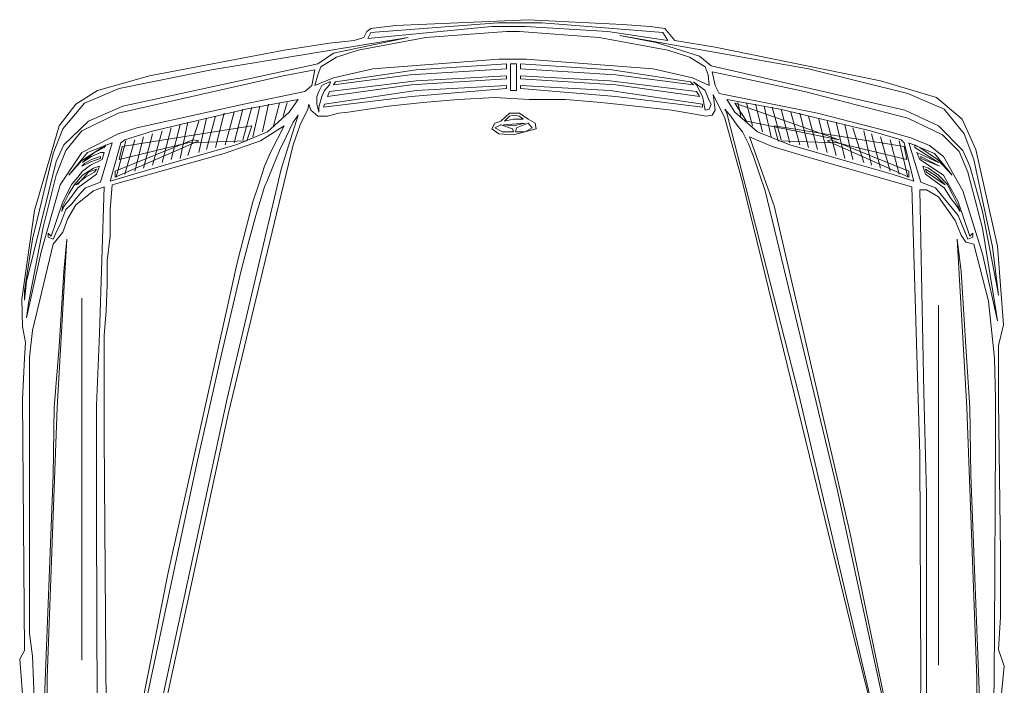
# Model space of a CAD drawing. Units: inches. Extents: x -9 to 646, y -802 to 47.
# Tile 9 of 17: x 432 to 486, y -561 to -525. Entities that reach past the tile are written whole.
import ezdxf

# ---------------------------------------------------------------- set-up
doc = ezdxf.new("R2010")
doc.units = ezdxf.units.IN
doc.header["$MEASUREMENT"] = 0
doc.layers.add('A-SITE-VEHI', color=8, linetype='Continuous', lineweight=9)

msp = doc.modelspace()

# ---------------------------------------------------------------- linework, layer by layer
at = {"layer": 'A-SITE-VEHI'}
for p, q in [((457.811, -525.081), (450.981, -525.732)), ((451.143, -525.408), (458.135, -524.866)), ((452.5, -525.028), (451.143, -525.19)), ((459.816, -524.701), (452.5, -525.028)), ((459.654, -525.081), (457.811, -525.081)), ((458.135, -524.866), (460.575, -524.866)), ((464.206, -525.352), (459.654, -525.081)), ((465.019, -524.974), (459.816, -524.701)), ((460.575, -524.866), (467.241, -525.408)), ((466.537, -525.081), (465.019, -524.974)), ((467.35, -525.19), (466.537, -525.081)), ((442.363, -527.466), (453.204, -525.678)), ((453.204, -525.678), (449.085, -526.544)), ((450.763, -525.678), (450.222, -525.841)), ((450.439, -526.382), (454.178, -525.678)), ((450.928, -525.352), (450.763, -525.678)), ((451.143, -525.19), (450.928, -525.352)), ((450.981, -525.732), (451.143, -525.408)), ((454.178, -525.678), (458.624, -525.352)), ((458.624, -525.352), (459.328, -525.352)), ((459.328, -525.352), (463.717, -525.678)), ((463.717, -525.678), (467.512, -526.382)), ((467.512, -525.841), (464.206, -525.352)), ((475.264, -527.413), (464.856, -525.57)), ((464.856, -525.57), (466.862, -525.949)), ((467.241, -525.408), (467.512, -525.841)), ((467.892, -525.841), (467.35, -525.19)), ((448.867, -526.003), (446.374, -526.382)), ((450.222, -525.841), (448.867, -526.003)), ((466.862, -525.949), (469.246, -526.709)), ((470.114, -526.22), (467.892, -525.841)), ((479.221, -528.063), (470.114, -526.22)), ((446.374, -526.382), (438.948, -527.792)), ((449.085, -526.544), (448.216, -527.142)), ((448.379, -527.304), (449.247, -526.762)), ((449.247, -526.762), (450.439, -526.382)), ((467.512, -526.382), (468.705, -526.762)), ((468.705, -526.762), (469.573, -527.304)), ((469.246, -526.709), (469.897, -527.25)), ((448.216, -527.142), (437.485, -529.473)), ((448.216, -527.737), (448.379, -527.304)), ((458.191, -526.871), (451.252, -527.413)), ((453.637, -527.466), (458.624, -527.142)), ((459.707, -526.871), (458.191, -526.871)), ((458.624, -527.142), (458.624, -527.413)), ((459.165, -527.142), (458.841, -527.142)), ((458.841, -527.142), (458.841, -528.605)), ((459.165, -528.605), (459.165, -527.142)), ((464.423, -527.466), (459.383, -527.142)), ((459.383, -527.142), (459.383, -527.413)), ((466.699, -527.413), (459.707, -526.871)), ((469.573, -527.304), (469.735, -527.737)), ((469.897, -527.25), (480.575, -529.689)), ((438.948, -527.792), (436.075, -528.605)), ((437.214, -529.851), (446.32, -527.792)), ((437.267, -528.496), (442.363, -527.466)), ((446.32, -527.792), (448.054, -527.466)), ((448.054, -527.466), (447.892, -528.334)), ((448.054, -528.334), (448.216, -527.737)), ((451.252, -527.413), (449.085, -527.901)), ((453.312, -527.737), (449.085, -528.281)), ((449.193, -528.116), (453.637, -527.466)), ((458.624, -527.413), (453.312, -527.737)), ((453.637, -528.063), (458.624, -527.792)), ((458.624, -527.792), (458.624, -527.954)), ((459.383, -527.413), (464.639, -527.737)), ((464.315, -528.063), (459.383, -527.792)), ((459.383, -527.792), (459.383, -527.954)), ((468.76, -528.116), (464.423, -527.466)), ((464.639, -527.737), (468.922, -528.281)), ((468.867, -527.901), (466.699, -527.413)), ((469.735, -527.737), (469.788, -528.334)), ((471.524, -527.901), (469.952, -527.575)), ((469.952, -527.575), (470.114, -528.334)), ((480.737, -528.767), (475.264, -527.413)), ((447.892, -528.334), (447.513, -528.658)), ((449.085, -527.901), (448.054, -528.334)), ((448.434, -528.334), (448.272, -528.658)), ((448.867, -528.116), (448.434, -528.334)), ((448.596, -528.605), (448.867, -528.281)), ((453.366, -528.281), (448.758, -528.929)), ((448.867, -528.658), (453.637, -528.063)), ((448.867, -528.281), (448.923, -528.116)), ((448.923, -528.116), (448.867, -528.116)), ((449.085, -528.281), (449.193, -528.116)), ((458.624, -527.954), (453.366, -528.281)), ((453.637, -528.605), (458.624, -528.334)), ((458.624, -528.334), (458.624, -528.496)), ((459.383, -527.954), (464.639, -528.281)), ((464.315, -528.605), (459.383, -528.334)), ((459.383, -528.334), (459.383, -528.496)), ((469.084, -528.658), (464.315, -528.063)), ((464.639, -528.281), (469.246, -528.929)), ((468.922, -528.281), (468.76, -528.116)), ((469.788, -528.334), (468.867, -527.901)), ((469.573, -528.605), (468.922, -528.116)), ((468.922, -528.116), (469.084, -528.281)), ((469.084, -528.281), (469.411, -528.929)), ((470.114, -528.334), (470.332, -528.767)), ((475.046, -528.658), (471.524, -527.901)), ((482.309, -528.985), (479.221, -528.063)), ((436.075, -528.605), (434.883, -529.364)), ((435.371, -529.309), (437.267, -528.496)), ((447.513, -528.658), (444.151, -529.364)), ((448.272, -528.658), (448.163, -528.929)), ((448.163, -528.929), (448.163, -529.364)), ((448.272, -529.526), (448.434, -528.929)), ((448.434, -528.929), (448.596, -528.605)), ((453.366, -528.929), (448.543, -529.526)), ((448.596, -529.364), (453.637, -528.605)), ((448.758, -528.929), (448.867, -528.658)), ((458.624, -528.496), (453.366, -528.929)), ((458.841, -528.605), (459.165, -528.605)), ((459.383, -528.496), (464.639, -528.929)), ((469.411, -529.364), (464.315, -528.605)), ((464.639, -528.929), (469.411, -529.526)), ((469.246, -528.929), (469.084, -528.658)), ((469.411, -528.929), (469.573, -529.689)), ((469.788, -529.147), (469.573, -528.605)), ((470.656, -530.122), (470.006, -528.823)), ((470.006, -528.823), (470.114, -529.689)), ((470.332, -528.767), (475.752, -529.851)), ((480.737, -530.122), (475.046, -528.658)), ((482.742, -529.635), (480.737, -528.767)), ((434.883, -529.364), (433.961, -530.557)), ((434.179, -530.719), (435.371, -529.309)), ((437.485, -529.473), (435.589, -530.286)), ((444.151, -529.364), (438.244, -530.666)), ((444.26, -529.635), (447.133, -529.093)), ((444.639, -531.152), (445.019, -529.473)), ((445.181, -530.881), (445.507, -529.364)), ((445.778, -530.557), (446.103, -529.309)), ((446.32, -530.015), (446.538, -529.256)), ((447.133, -529.093), (446.644, -529.797)), ((447.73, -529.364), (447.675, -529.635)), ((447.837, -529.689), (447.73, -529.364)), ((448.163, -529.364), (448.272, -529.797)), ((448.543, -529.526), (448.596, -529.364)), ((452.12, -529.473), (449.897, -529.797)), ((454.016, -529.256), (452.12, -529.473)), ((455.968, -529.093), (454.016, -529.256)), ((457.973, -528.985), (455.968, -529.093)), ((459.869, -529.093), (457.973, -528.985)), ((461.877, -529.093), (459.869, -529.093)), ((463.826, -529.256), (461.877, -529.093)), ((465.725, -529.473), (463.826, -529.256)), ((467.73, -529.689), (465.725, -529.473)), ((469.411, -529.526), (469.411, -529.364)), ((469.897, -529.364), (469.788, -529.147)), ((469.788, -529.635), (469.897, -529.364)), ((473.692, -529.635), (470.765, -529.093)), ((470.765, -529.093), (471.198, -529.797)), ((476.945, -531.314), (471.198, -529.309)), ((471.198, -529.309), (471.849, -530.286)), ((471.524, -530.015), (471.36, -529.256)), ((472.173, -530.557), (471.849, -529.309)), ((472.717, -530.881), (472.337, -529.364)), ((473.203, -531.152), (472.823, -529.473)), ((483.719, -530.177), (482.309, -528.985)), ((435.209, -530.828), (437.214, -529.851)), ((439.166, -530.828), (444.26, -529.635)), ((442.092, -531.858), (442.581, -530.015)), ((442.581, -531.749), (443.067, -529.851)), ((443.123, -531.587), (443.609, -529.797)), ((443.609, -531.478), (444.098, -529.635)), ((444.098, -531.314), (444.586, -529.526)), ((446.644, -529.797), (445.452, -530.881)), ((446.211, -532.941), (447.133, -529.959)), ((447.133, -529.959), (446.862, -530.339)), ((447.675, -529.635), (447.242, -530.501)), ((448.216, -530.015), (447.837, -529.689)), ((448.758, -530.015), (448.216, -530.015)), ((448.272, -529.797), (448.272, -529.526)), ((449.356, -529.851), (448.758, -530.015)), ((449.897, -529.797), (449.356, -529.851)), ((458.786, -529.851), (458.297, -530.286)), ((458.786, -530.015), (458.515, -530.286)), ((459.328, -529.851), (458.786, -529.851)), ((459.003, -529.959), (458.786, -530.015)), ((459.328, -530.015), (459.003, -529.959)), ((459.816, -530.177), (459.328, -529.851)), ((459.545, -530.177), (459.328, -530.015)), ((469.626, -530.015), (467.73, -529.689)), ((469.573, -529.689), (469.788, -529.635)), ((469.952, -529.959), (469.626, -530.015)), ((470.114, -529.689), (469.952, -529.959)), ((470.981, -530.015), (470.656, -529.635)), ((470.656, -529.635), (470.765, -529.851)), ((470.765, -529.851), (474.722, -545.354)), ((471.307, -530.501), (470.981, -530.015)), ((471.198, -529.797), (472.444, -530.881)), ((473.745, -531.314), (473.259, -529.526)), ((478.679, -530.828), (473.692, -529.635)), ((474.233, -531.478), (473.745, -529.635)), ((474.775, -531.587), (474.287, -529.797)), ((475.264, -531.749), (474.775, -529.851)), ((475.752, -531.858), (475.264, -530.015)), ((475.752, -529.851), (479.545, -530.828)), ((480.575, -529.689), (482.418, -530.557)), ((483.828, -530.99), (482.742, -529.635)), ((433.961, -530.557), (432.607, -535.217)), ((435.589, -530.286), (434.232, -531.587)), ((437.432, -531.694), (444.586, -530.557)), ((440.141, -532.4), (440.629, -530.501)), ((440.629, -532.344), (441.062, -530.339)), ((441.062, -532.182), (441.659, -530.286)), ((441.659, -532.02), (442.092, -530.122)), ((444.586, -530.557), (444.315, -531.369)), ((446.374, -530.557), (445.072, -531.369)), ((445.616, -532.02), (446.374, -530.557)), ((446.862, -530.339), (446.482, -531.152)), ((447.242, -530.501), (446.862, -531.587)), ((457.973, -530.395), (457.811, -530.719)), ((458.297, -530.286), (457.973, -530.395)), ((458.297, -530.501), (457.973, -530.666)), ((458.948, -530.719), (458.297, -530.501)), ((459.654, -530.395), (458.462, -530.501)), ((458.462, -530.501), (459.003, -530.557)), ((458.515, -530.286), (459.003, -530.177)), ((459.003, -530.177), (459.545, -530.177)), ((459.003, -530.557), (459.654, -530.395)), ((459.816, -530.395), (459.165, -530.666)), ((460.196, -530.395), (459.816, -530.177)), ((460.034, -530.666), (459.816, -530.395)), ((460.249, -530.719), (460.196, -530.395)), ((471.631, -533.645), (470.656, -530.122)), ((471.631, -530.881), (471.307, -530.501)), ((471.849, -530.286), (476.945, -531.314)), ((480.522, -531.694), (473.365, -530.557)), ((473.365, -530.557), (473.583, -531.369)), ((476.294, -532.02), (475.806, -530.122)), ((476.78, -532.182), (476.294, -530.286)), ((477.269, -532.344), (476.78, -530.339)), ((477.702, -532.4), (477.269, -530.501)), ((482.636, -531.043), (480.737, -530.122)), ((482.418, -530.557), (483.772, -531.911)), ((484.479, -531.858), (483.719, -530.177)), ((433.637, -532.073), (434.179, -530.719)), ((434.341, -531.911), (435.209, -530.828)), ((437.214, -530.99), (435.209, -532.02)), ((438.244, -530.666), (437.214, -530.99)), ((437.594, -531.314), (439.166, -530.828)), ((438.624, -532.886), (439.11, -530.99)), ((439.11, -532.724), (439.652, -530.828)), ((439.652, -532.562), (440.141, -530.666)), ((445.452, -530.881), (443.718, -531.587)), ((457.811, -530.719), (458.191, -530.99)), ((457.973, -530.666), (458.406, -530.881)), ((458.191, -530.99), (459.003, -531.043)), ((458.406, -530.881), (459.003, -530.881)), ((459.003, -530.881), (458.948, -530.719)), ((459.003, -531.043), (460.249, -530.719)), ((459.165, -530.666), (459.112, -530.881)), ((459.112, -530.881), (459.654, -530.881)), ((459.654, -530.881), (460.034, -530.666)), ((471.957, -531.532), (471.631, -530.881)), ((472.444, -530.881), (474.233, -531.587)), ((478.299, -532.562), (477.702, -530.666)), ((478.732, -532.724), (478.299, -530.828)), ((480.357, -531.314), (478.679, -530.828)), ((479.221, -532.886), (478.732, -530.99)), ((479.545, -530.828), (480.899, -531.207)), ((483.557, -531.965), (482.636, -531.043)), ((484.37, -532.4), (483.828, -530.99)), ((434.232, -531.587), (433.799, -532.506)), ((435.533, -532.02), (436.89, -531.478)), ((436.89, -531.478), (436.239, -533.645)), ((436.564, -531.587), (436.346, -531.749)), ((436.455, -531.749), (436.564, -531.587)), ((436.781, -533.592), (437.376, -531.478)), ((437.052, -533.05), (441.333, -531.314)), ((441.659, -531.369), (437.052, -533.374)), ((437.105, -533.374), (437.647, -531.369)), ((441.062, -531.478), (437.267, -532.4)), ((437.376, -531.478), (437.594, -531.314)), ((437.594, -533.212), (438.136, -531.314)), ((438.136, -533.05), (438.624, -531.152)), ((443.718, -531.587), (440.467, -532.506)), ((444.315, -531.369), (441.062, -531.478)), ((441.333, -531.314), (441.659, -531.369)), ((445.072, -531.369), (443.067, -532.073)), ((446.862, -531.587), (443.285, -546.437)), ((446.482, -531.152), (446.103, -531.911)), ((472.228, -532.235), (471.957, -531.532)), ((473.259, -531.694), (472.011, -531.152)), ((472.011, -531.152), (473.365, -534.947)), ((473.583, -531.369), (476.836, -531.478)), ((474.233, -531.587), (477.431, -532.506)), ((476.509, -531.314), (476.294, -531.369)), ((476.294, -531.369), (480.793, -533.374)), ((480.793, -533.05), (476.509, -531.314)), ((476.836, -531.478), (480.684, -532.4)), ((479.762, -533.05), (479.221, -531.152)), ((480.251, -533.212), (479.762, -531.314)), ((480.737, -533.374), (480.251, -531.369)), ((480.522, -531.478), (480.357, -531.314)), ((481.064, -533.592), (480.522, -531.478)), ((482.2, -532.073), (480.793, -531.478)), ((480.793, -531.478), (481.443, -533.645)), ((480.899, -531.207), (481.93, -531.64)), ((481.117, -531.749), (481.117, -531.587)), ((481.117, -531.587), (481.388, -531.749)), ((481.93, -531.64), (482.689, -532.235)), ((432.498, -536.79), (433.637, -532.073)), ((433.799, -533.266), (434.341, -531.911)), ((435.209, -532.02), (434.017, -533.808)), ((434.503, -533.266), (435.533, -532.02)), ((436.346, -531.749), (435.209, -532.453)), ((435.751, -532.235), (435.262, -532.562)), ((435.425, -532.4), (435.913, -532.02)), ((436.239, -532.02), (435.751, -532.235)), ((435.751, -532.4), (436.239, -532.235)), ((435.913, -532.02), (436.455, -531.749)), ((436.455, -532.02), (436.239, -532.02)), ((436.239, -532.235), (436.239, -532.344)), ((436.346, -532.4), (436.455, -532.02)), ((443.067, -532.073), (436.89, -533.808)), ((437.267, -532.4), (437.432, -531.694)), ((445.29, -532.779), (445.616, -532.02)), ((446.103, -531.911), (445.778, -532.724)), ((472.553, -533.212), (472.228, -532.235)), ((475.479, -532.344), (473.259, -531.694)), ((480.684, -532.4), (480.522, -531.694)), ((482.418, -532.562), (481.117, -531.749)), ((481.388, -532.4), (481.226, -532.02)), ((481.226, -532.02), (482.418, -532.562)), ((481.388, -531.749), (482.365, -532.4)), ((481.443, -532.235), (481.443, -532.344)), ((482.471, -532.779), (481.443, -532.235)), ((483.177, -533.266), (482.2, -532.073)), ((482.689, -532.235), (483.772, -534.134)), ((484.043, -533.104), (483.557, -531.965)), ((483.772, -531.911), (484.152, -532.779)), ((485.671, -537.169), (484.479, -531.858)), ((433.799, -532.506), (432.174, -539.121)), ((435.209, -532.453), (434.503, -533.266)), ((435.751, -532.506), (435.209, -532.779)), ((435.209, -532.779), (435.371, -532.615)), ((435.262, -532.562), (435.425, -532.4)), ((435.262, -533.05), (435.698, -532.724)), ((435.371, -532.615), (435.751, -532.4)), ((435.698, -532.724), (436.346, -532.4)), ((436.239, -532.344), (435.751, -532.506)), ((440.467, -532.506), (438.082, -533.212)), ((445.778, -532.724), (445.452, -533.537)), ((480.955, -533.916), (475.479, -532.344)), ((477.431, -532.506), (479.871, -533.212)), ((482.689, -533.266), (481.388, -532.4)), ((481.443, -532.344), (482.471, -532.779)), ((482.365, -532.4), (483.177, -533.266)), ((485.398, -537.223), (484.37, -532.4)), ((433.095, -536.139), (433.799, -533.266)), ((434.829, -533.754), (435.262, -533.266)), ((434.991, -533.374), (435.262, -533.05)), ((434.991, -533.754), (435.589, -533.104)), ((436.022, -533.212), (434.991, -533.972)), ((435.262, -533.266), (435.86, -532.886)), ((435.913, -533.104), (435.425, -533.374)), ((435.589, -533.104), (436.022, -532.941)), ((435.86, -532.886), (436.184, -532.779)), ((436.022, -532.941), (435.913, -533.104)), ((436.184, -532.779), (436.022, -533.212)), ((438.082, -533.212), (436.781, -533.592)), ((437.052, -533.374), (437.052, -533.05)), ((443.232, -545.569), (446.211, -532.941)), ((444.966, -533.754), (445.29, -532.779)), ((472.879, -534.134), (472.553, -533.212)), ((479.871, -533.212), (481.064, -533.592)), ((480.793, -533.374), (480.793, -533.05)), ((481.876, -532.886), (481.55, -532.779)), ((481.55, -532.779), (481.714, -533.212)), ((482.309, -533.321), (481.714, -532.941)), ((481.714, -532.941), (481.767, -533.104)), ((481.714, -533.212), (482.742, -533.972)), ((481.767, -533.104), (482.798, -533.808)), ((482.418, -533.266), (481.876, -532.886)), ((482.906, -533.754), (482.418, -533.266)), ((483.502, -534.729), (482.689, -533.266)), ((484.856, -536.192), (484.043, -533.104)), ((484.152, -532.779), (484.856, -535.271)), ((434.017, -533.808), (432.986, -537.493)), ((434.179, -534.729), (434.667, -533.754)), ((434.503, -534.296), (434.829, -533.754)), ((434.667, -533.754), (434.991, -533.374)), ((435.425, -533.374), (434.883, -533.808)), ((434.883, -533.808), (434.991, -533.754)), ((435.86, -533.808), (435.425, -533.972)), ((436.239, -533.645), (435.86, -533.808)), ((436.89, -533.808), (436.781, -535.164)), ((444.639, -534.729), (444.966, -533.754)), ((445.452, -533.537), (445.29, -533.916)), ((474.287, -544.541), (471.631, -533.645)), ((481.443, -533.645), (482.256, -533.972)), ((482.798, -533.808), (482.309, -533.321)), ((483.177, -534.296), (482.906, -533.754)), ((434.179, -534.947), (434.503, -534.296)), ((434.991, -533.972), (434.558, -534.567)), ((435.86, -534.134), (434.883, -534.893)), ((435.154, -534.243), (434.883, -534.567)), ((435.425, -533.972), (435.154, -534.243)), ((436.455, -533.916), (435.86, -534.134)), ((436.184, -541.992), (436.455, -533.916)), ((445.29, -533.916), (444.801, -535.488)), ((476.836, -550.556), (472.879, -534.134)), ((481.388, -548.66), (480.955, -533.916)), ((481.767, -534.078), (481.388, -534.078)), ((481.388, -534.078), (481.605, -545.245)), ((482.418, -534.458), (481.767, -534.078)), ((482.256, -533.972), (483.502, -535.488)), ((482.742, -533.972), (483.122, -534.567)), ((483.502, -534.947), (483.177, -534.296)), ((483.772, -534.134), (484.856, -537.602)), ((433.799, -535.815), (434.179, -534.729)), ((434.125, -535.271), (434.179, -534.947)), ((434.558, -534.567), (434.232, -535)), ((434.667, -534.838), (434.341, -535.164)), ((434.883, -534.893), (434.45, -535.65)), ((434.883, -534.567), (434.667, -534.838)), ((444.315, -536.03), (444.639, -534.729)), ((473.365, -534.947), (477.54, -552.941)), ((483.339, -535.759), (482.418, -534.458)), ((483.122, -534.567), (483.448, -535)), ((484.152, -536.627), (483.502, -534.729)), ((483.61, -535.271), (483.502, -534.947)), ((432.607, -535.217), (431.903, -540.096)), ((434.232, -535), (434.125, -535.271)), ((434.341, -535.164), (434.179, -535.597)), ((436.781, -535.164), (436.781, -536.627)), ((444.801, -535.488), (444.424, -536.898)), ((483.448, -535), (483.61, -535.271)), ((483.502, -535.488), (484.043, -536.79)), ((484.856, -535.271), (485.671, -539.554)), ((433.528, -536.627), (433.799, -535.815)), ((434.017, -535.977), (433.855, -536.301)), ((434.179, -535.597), (434.017, -535.977)), ((434.45, -535.65), (434.179, -536.41)), ((443.773, -538.091), (444.315, -536.03)), ((483.664, -536.572), (483.339, -535.759)), ((432.283, -540.313), (433.095, -536.139)), ((433.366, -536.681), (433.366, -536.463)), ((433.366, -536.463), (433.528, -536.627)), ((433.855, -536.301), (433.637, -536.79)), ((434.179, -536.41), (433.637, -537.06)), ((483.935, -536.952), (483.664, -536.572)), ((484.314, -536.463), (484.152, -536.627)), ((484.314, -536.681), (484.314, -536.463)), ((485.562, -540.584), (484.856, -536.192)), ((432.118, -539.283), (432.498, -536.79)), ((433.637, -537.06), (432.498, -541.83)), ((433.637, -536.79), (433.366, -536.681)), ((433.855, -546.058), (434.396, -536.79)), ((434.396, -536.79), (434.232, -538.577)), ((436.781, -536.627), (436.617, -537.982)), ((444.424, -536.898), (443.989, -538.524)), ((483.99, -546.058), (483.448, -536.79)), ((483.448, -536.79), (483.664, -538.577)), ((484.37, -537.06), (483.935, -536.952)), ((484.043, -536.79), (484.314, -536.681)), ((485.182, -540.205), (484.37, -537.06)), ((432.986, -537.493), (432.174, -541.126)), ((484.856, -537.602), (485.671, -541.288)), ((485.724, -539.878), (485.398, -537.223)), ((485.995, -541.506), (485.671, -537.169)), ((436.617, -537.982), (436.617, -539.283)), ((443.232, -540.584), (443.773, -538.091)), ((434.232, -538.577), (433.961, -542.698)), ((443.989, -538.524), (442.905, -543.131)), ((483.664, -538.577), (483.935, -542.698)), ((432.174, -539.121), (432.065, -540.149)), ((432.065, -539.663), (432.118, -539.283)), ((436.617, -539.283), (436.564, -540.746)), ((432.065, -540.149), (432.065, -539.663)), ((485.671, -539.554), (485.724, -539.878)), ((431.903, -540.096), (431.956, -541.612)), ((432.174, -541.126), (432.283, -540.313)), ((435.209, -559.987), (435.209, -540.04)), ((485.507, -543.347), (485.182, -540.205)), ((436.564, -540.746), (436.455, -542.101)), ((439.979, -555.164), (443.232, -540.584)), ((482.418, -560.257), (482.418, -540.42)), ((485.671, -541.288), (485.562, -540.584)), ((431.956, -541.612), (432.118, -542.481)), ((432.498, -541.83), (432.336, -543.293)), ((436.022, -545.949), (436.184, -541.992)), ((485.724, -542.643), (485.995, -541.506)), ((432.118, -542.481), (432.065, -543.347)), ((436.455, -542.101), (436.455, -547.63)), ((433.961, -542.698), (433.69, -546.058)), ((483.935, -542.698), (484.152, -546.058)), ((485.724, -545.733), (485.724, -542.643)), ((432.065, -543.347), (431.956, -545.625)), ((432.336, -543.293), (432.336, -558.523)), ((442.905, -543.131), (441.551, -549.146)), ((485.562, -545.569), (485.507, -543.347)), ((477.811, -558.958), (474.287, -544.541)), ((481.605, -545.245), (481.767, -550.827)), ((431.956, -545.625), (432.065, -559.445)), ((438.84, -565.895), (443.232, -545.569)), ((474.722, -545.354), (479.383, -565.082)), ((485.562, -547.792), (485.562, -545.569)), ((485.833, -554.08), (485.724, -545.733)), ((433.311, -560.964), (433.855, -546.058)), ((433.69, -546.058), (433.637, -549.797)), ((436.022, -552.237), (436.022, -545.949)), ((484.532, -560.964), (483.99, -546.058)), ((484.152, -546.058), (484.206, -549.797)), ((443.285, -546.437), (439.652, -563.186)), ((436.455, -547.63), (436.564, -563.186)), ((485.507, -558.523), (485.562, -547.792)), ((481.443, -560.855), (481.388, -548.66)), ((441.551, -549.146), (438.244, -564.703)), ((433.637, -549.797), (433.149, -562.536)), ((484.206, -549.797), (484.694, -562.536)), ((480.522, -567.521), (476.836, -550.556)), ((481.767, -550.827), (481.767, -569.039)), ((436.075, -564.756), (436.022, -552.237)), ((477.54, -552.941), (480.522, -567.25)), ((485.833, -557.602), (485.833, -554.08)), ((438.082, -564.703), (439.979, -555.164)), ((485.724, -559.391), (485.833, -557.602)), ((432.336, -558.523), (432.498, -559.771)), ((485.398, -568.984), (485.507, -558.523)), ((479.383, -565.082), (477.811, -558.958)), ((432.065, -559.445), (431.794, -559.933)), ((432.498, -559.771), (432.607, -562.48)), ((486.048, -560.313), (485.724, -559.391)), ((431.794, -559.933), (432.065, -563.239)), ((485.886, -561.83), (486.048, -560.313)), ((433.311, -568.984), (433.311, -560.964)), ((481.388, -568.551), (481.443, -560.855)), ((484.532, -568.984), (484.532, -560.964))]:
    msp.add_line(p, q, dxfattribs=at)

doc.saveas('drawing.dxf')
